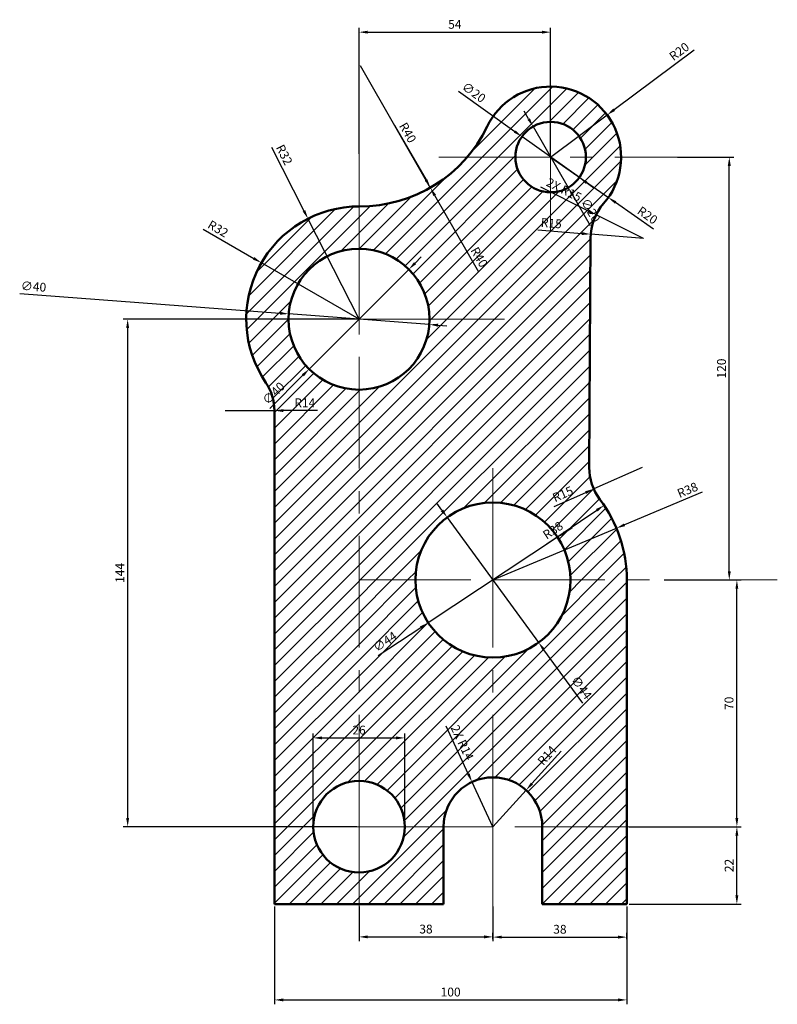
# Model space of a CAD drawing. Units: millimetres. Extents: x 2125 to 2340, y 1172 to 1452.
import ezdxf

# ---------------------------------------------------------------- set-up
doc = ezdxf.new("R2010")
doc.units = ezdxf.units.MM
doc.linetypes.add('CENTER', pattern=[50.8, 31.75, -6.35, 6.35, -6.35])
for name, color, linetype, lineweight in [('M-CNTR', 4, 'CENTER', 18), ('M-DIMS', 2, 'Continuous', 25), ('M-HATC', 8, 'Continuous', 18), ('M-OUTL', 7, 'Continuous', 50)]:
    doc.layers.add(name, color=color, linetype=linetype, lineweight=lineweight)
doc.styles.get("Standard").update_dxf_attribs({"font": 'arial.ttf'})
doc.dimstyles.new('ISO-25', dxfattribs={"dimtxt": 2.5, "dimasz": 2.5, "dimexe": 1.25, "dimexo": 0.625, "dimtad": 1, "dimdec": 0, "dimtxsty": 'Standard', "dimcen": 2.5, "dimadec": 0, "dimazin": 0, "dimtfac": 1, "dimtdec": 0, "dimtmove": 0, "dimatfit": 3, "dimfxl": 1, "dimarcsym": 0})

# ---------------------------------------------------------------- blocks, each defined once
blk = doc.blocks.new('*D1')
at = {"layer": 'Defpoints', "color": 0, "transparency": 16777216}
for p in [(2311.5, 1412.62), (2326.85, 1412.62), (2311.5, 1292.62)]:
    blk.add_point(p, dxfattribs=at)
at = {"layer": 'M-DIMS', "color": 0, "lineweight": -2, "transparency": 16777216}
for p, q in [((2312.12, 1412.62), (2328.1, 1412.62)), ((2326.85, 1295.12), (2326.85, 1410.12)), ((2312.12, 1292.62), (2328.1, 1292.62))]:
    blk.add_line(p, q, dxfattribs=at)
at = {"layer": 'M-DIMS', "color": 0, "transparency": 16777216}
for points in [[(2326.43, 1410.12), (2327.27, 1410.12), (2326.85, 1412.62)], [(2326.43, 1295.12), (2327.27, 1295.12), (2326.85, 1292.62)]]:
    blk.add_solid(points, dxfattribs=at)
at = {"layer": 'M-DIMS', "color": 0, "transparency": 16777216, "insert": (2324.95, 1352.62), "char_height": 2.5, "attachment_point": 5, "rotation": 90}
blk.add_mtext('120', dxfattribs=at)
blk = doc.blocks.new('*D2')
at = {"layer": 'Defpoints', "color": 0, "transparency": 16777216}
for p in [(2276.15, 1448.06), (2221.77, 1412.88), (2276.15, 1412.62)]:
    blk.add_point(p, dxfattribs=at)
at = {"layer": 'M-DIMS', "color": 0, "lineweight": -2, "transparency": 16777216}
for p, q in [((2221.77, 1413.51), (2221.77, 1449.31)), ((2224.27, 1448.06), (2273.65, 1448.06)), ((2276.15, 1413.24), (2276.15, 1449.31))]:
    blk.add_line(p, q, dxfattribs=at)
at = {"layer": 'M-DIMS', "color": 0, "transparency": 16777216}
for points in [[(2224.27, 1448.48), (2224.27, 1447.65), (2221.77, 1448.06)], [(2273.65, 1448.48), (2273.65, 1447.65), (2276.15, 1448.06)]]:
    blk.add_solid(points, dxfattribs=at)
at = {"layer": 'M-DIMS', "color": 0, "transparency": 16777216, "insert": (2248.96, 1449.96), "char_height": 2.5, "attachment_point": 5}
blk.add_mtext('54', dxfattribs=at)
blk = doc.blocks.new('*D3')
at = {"layer": 'Defpoints', "color": 0, "transparency": 16777216}
for p in [(2307.75, 1292.62), (2329, 1292.62), (2307.75, 1222.62)]:
    blk.add_point(p, dxfattribs=at)
at = {"layer": 'M-DIMS', "color": 0, "lineweight": -2, "transparency": 16777216}
for p, q in [((2308.38, 1292.62), (2330.25, 1292.62)), ((2329, 1225.12), (2329, 1290.12)), ((2308.38, 1222.62), (2330.25, 1222.62))]:
    blk.add_line(p, q, dxfattribs=at)
at = {"layer": 'M-DIMS', "color": 0, "transparency": 16777216}
for points in [[(2328.58, 1290.12), (2329.41, 1290.12), (2329, 1292.62)], [(2328.58, 1225.12), (2329.41, 1225.12), (2329, 1222.62)]]:
    blk.add_solid(points, dxfattribs=at)
at = {"layer": 'M-DIMS', "color": 0, "transparency": 16777216, "insert": (2327.09, 1257.62), "char_height": 2.5, "attachment_point": 5, "rotation": 90}
blk.add_mtext('70', dxfattribs=at)
blk = doc.blocks.new('*D4')
at = {"layer": 'Defpoints', "color": 0, "transparency": 16777216}
for p in [(2297.77, 1222.62), (2329, 1222.62), (2297.77, 1200.62)]:
    blk.add_point(p, dxfattribs=at)
at = {"layer": 'M-DIMS', "color": 0, "lineweight": -2, "transparency": 16777216}
for p, q in [((2298.39, 1222.62), (2330.25, 1222.62)), ((2329, 1203.12), (2329, 1220.12)), ((2298.39, 1200.62), (2330.25, 1200.62))]:
    blk.add_line(p, q, dxfattribs=at)
at = {"layer": 'M-DIMS', "color": 0, "transparency": 16777216}
for points in [[(2328.58, 1220.12), (2329.41, 1220.12), (2329, 1222.62)], [(2328.58, 1203.12), (2329.41, 1203.12), (2329, 1200.62)]]:
    blk.add_solid(points, dxfattribs=at)
at = {"layer": 'M-DIMS', "color": 0, "transparency": 16777216, "insert": (2327.12, 1211.62), "char_height": 2.5, "attachment_point": 5, "rotation": 90}
blk.add_mtext('22', dxfattribs=at)
blk = doc.blocks.new('*D5')
at = {"layer": 'Defpoints', "color": 0, "transparency": 16777216}
for p in [(2221.77, 1366.62), (2156.11, 1222.62), (2221.77, 1222.62)]:
    blk.add_point(p, dxfattribs=at)
at = {"layer": 'M-DIMS', "color": 0, "lineweight": -2, "transparency": 16777216}
for p, q in [((2221.14, 1366.62), (2154.86, 1366.62)), ((2156.11, 1364.12), (2156.11, 1225.12)), ((2221.14, 1222.62), (2154.86, 1222.62))]:
    blk.add_line(p, q, dxfattribs=at)
at = {"layer": 'M-DIMS', "color": 0, "transparency": 16777216}
for points in [[(2155.69, 1364.12), (2156.53, 1364.12), (2156.11, 1366.62)], [(2155.69, 1225.12), (2156.53, 1225.12), (2156.11, 1222.62)]]:
    blk.add_solid(points, dxfattribs=at)
at = {"layer": 'M-DIMS', "color": 0, "transparency": 16777216, "insert": (2154.23, 1294.62), "char_height": 2.5, "attachment_point": 5, "rotation": 90}
blk.add_mtext('144', dxfattribs=at)
blk = doc.blocks.new('*D6')
at = {"layer": 'Defpoints', "color": 0, "transparency": 16777216}
for p in [(2234.77, 1247.81), (2208.77, 1222.62), (2234.77, 1222.62)]:
    blk.add_point(p, dxfattribs=at)
at = {"layer": 'M-DIMS', "color": 0, "lineweight": -2, "transparency": 16777216}
for p, q in [((2208.77, 1223.24), (2208.77, 1249.06)), ((2234.77, 1223.24), (2234.77, 1249.06)), ((2211.27, 1247.81), (2232.27, 1247.81))]:
    blk.add_line(p, q, dxfattribs=at)
at = {"layer": 'M-DIMS', "color": 0, "transparency": 16777216}
for points in [[(2211.27, 1248.23), (2211.27, 1247.4), (2208.77, 1247.81)], [(2232.27, 1248.23), (2232.27, 1247.4), (2234.77, 1247.81)]]:
    blk.add_solid(points, dxfattribs=at)
at = {"layer": 'M-DIMS', "color": 0, "transparency": 16777216, "insert": (2221.77, 1249.71), "char_height": 2.5, "attachment_point": 5}
blk.add_mtext('26', dxfattribs=at)
blk = doc.blocks.new('*D7')
at = {"layer": 'Defpoints', "color": 0, "transparency": 16777216}
for p in [(2292.19, 1424.57), (2276.15, 1412.62)]:
    blk.add_point(p, dxfattribs=at)
at = {"layer": 'M-DIMS', "color": 0, "lineweight": -2, "transparency": 16777216}
for p, q in [((2316.85, 1442.95), (2294.19, 1426.06)), ((2276.15, 1412.62), (2292.19, 1424.57))]:
    blk.add_line(p, q, dxfattribs=at)
at = {"layer": 'M-DIMS', "color": 0, "transparency": 16777216}
blk.add_solid([(2293.94, 1426.4), (2294.44, 1425.73), (2292.19, 1424.57)], dxfattribs=at)
at = {"layer": 'M-DIMS', "color": 0, "transparency": 16777216, "insert": (2312.82, 1442.32), "char_height": 2.5, "attachment_point": 5, "rotation": 36.702}
blk.add_mtext('R20', dxfattribs=at)
blk = doc.blocks.new('*D8')
at = {"layer": 'Defpoints', "color": 0, "transparency": 16777216}
for p in [(2222.08, 1438.62), (2242.03, 1403.95)]:
    blk.add_point(p, dxfattribs=at)
at = {"layer": 'M-DIMS', "color": 0, "lineweight": -2, "transparency": 16777216}
blk.add_line((2231.88, 1421.58), (2240.79, 1406.12), dxfattribs=at)
at = {"layer": 'M-DIMS', "color": 0, "transparency": 16777216}
blk.add_solid([(2241.15, 1406.32), (2240.43, 1405.91), (2242.03, 1403.95)], dxfattribs=at)
at = {"layer": 'M-DIMS', "color": 0, "transparency": 16777216, "insert": (2235.33, 1419.4), "char_height": 2.5, "attachment_point": 5, "rotation": 299.9242}
blk.add_mtext('R40', dxfattribs=at)
blk = doc.blocks.new('*D9')
at = {"layer": 'Defpoints', "color": 0, "transparency": 16777216}
for p in [(2287.51, 1390.73), (2302.46, 1389.53)]:
    blk.add_point(p, dxfattribs=at)
at = {"layer": 'M-DIMS', "color": 0, "lineweight": -2, "transparency": 16777216}
for p, q in [((2272.54, 1391.93), (2285.02, 1390.93)), ((2302.46, 1389.53), (2287.51, 1390.73))]:
    blk.add_line(p, q, dxfattribs=at)
at = {"layer": 'M-DIMS', "color": 0, "transparency": 16777216}
blk.add_solid([(2285.05, 1391.34), (2284.98, 1390.51), (2287.51, 1390.73)], dxfattribs=at)
at = {"layer": 'M-DIMS', "color": 0, "transparency": 16777216, "insert": (2276.31, 1393.53), "char_height": 2.5, "attachment_point": 5, "rotation": 355.4193}
blk.add_mtext('R15', dxfattribs=at)
blk = doc.blocks.new('*D10')
at = {"layer": 'Defpoints', "color": 0, "transparency": 16777216}
for p in [(2302.1, 1324.5), (2288.38, 1318.44)]:
    blk.add_point(p, dxfattribs=at)
at = {"layer": 'M-DIMS', "color": 0, "lineweight": -2, "transparency": 16777216}
for p, q in [((2302.1, 1324.5), (2288.38, 1318.44)), ((2277.18, 1313.5), (2286.1, 1317.43))]:
    blk.add_line(p, q, dxfattribs=at)
at = {"layer": 'M-DIMS', "color": 0, "transparency": 16777216}
blk.add_solid([(2285.93, 1317.81), (2286.26, 1317.05), (2288.38, 1318.44)], dxfattribs=at)
at = {"layer": 'M-DIMS', "color": 0, "transparency": 16777216, "insert": (2279.73, 1316.7), "char_height": 2.5, "attachment_point": 5, "rotation": 23.827}
blk.add_mtext('R15', dxfattribs=at)
blk = doc.blocks.new('*D11')
at = {"layer": 'Defpoints', "color": 0, "transparency": 16777216}
for p in [(2291.32, 1313.8), (2259.77, 1292.62)]:
    blk.add_point(p, dxfattribs=at)
at = {"layer": 'M-DIMS', "color": 0, "lineweight": -2, "transparency": 16777216}
blk.add_line((2275.03, 1302.86), (2289.24, 1312.4), dxfattribs=at)
at = {"layer": 'M-DIMS', "color": 0, "transparency": 16777216}
blk.add_solid([(2289.01, 1312.75), (2289.48, 1312.06), (2291.32, 1313.8)], dxfattribs=at)
at = {"layer": 'M-DIMS', "color": 0, "transparency": 16777216, "insert": (2276.97, 1306.46), "char_height": 2.5, "attachment_point": 5, "rotation": 33.8706}
blk.add_mtext('R38', dxfattribs=at)
blk = doc.blocks.new('*D12')
at = {"layer": 'Defpoints', "color": 0, "transparency": 16777216}
for p in [(2194.06, 1382.62), (2221.77, 1366.62)]:
    blk.add_point(p, dxfattribs=at)
at = {"layer": 'M-DIMS', "color": 0, "lineweight": -2, "transparency": 16777216}
for p, q in [((2177.53, 1392.16), (2191.89, 1383.87)), ((2221.77, 1366.62), (2194.06, 1382.62))]:
    blk.add_line(p, q, dxfattribs=at)
at = {"layer": 'M-DIMS', "color": 0, "transparency": 16777216}
blk.add_solid([(2192.1, 1384.23), (2191.68, 1383.51), (2194.06, 1382.62)], dxfattribs=at)
at = {"layer": 'M-DIMS', "color": 0, "transparency": 16777216, "insert": (2181.6, 1392), "char_height": 2.5, "attachment_point": 5, "rotation": 330}
blk.add_mtext('R32', dxfattribs=at)
blk = doc.blocks.new('*D13')
at = {"layer": 'Defpoints', "color": 0, "transparency": 16777216}
for p in [(2183.77, 1340.69), (2197.77, 1340.69)]:
    blk.add_point(p, dxfattribs=at)
at = {"layer": 'M-DIMS', "color": 0, "lineweight": -2, "transparency": 16777216}
for p, q in [((2183.77, 1340.69), (2197.77, 1340.69)), ((2209.98, 1340.69), (2200.27, 1340.69))]:
    blk.add_line(p, q, dxfattribs=at)
at = {"layer": 'M-DIMS', "color": 0, "transparency": 16777216}
blk.add_solid([(2200.27, 1341.11), (2200.27, 1340.28), (2197.77, 1340.69)], dxfattribs=at)
at = {"layer": 'M-DIMS', "color": 0, "transparency": 16777216, "insert": (2206.38, 1342.57), "char_height": 2.5, "attachment_point": 5}
blk.add_mtext('R14', dxfattribs=at)
blk = doc.blocks.new('*D14')
at = {"layer": 'Defpoints', "color": 0, "transparency": 16777216}
for p in [(2269.17, 1232.99), (2259.77, 1222.62)]:
    blk.add_point(p, dxfattribs=at)
at = {"layer": 'M-DIMS', "color": 0, "lineweight": -2, "transparency": 16777216}
for p, q in [((2279.17, 1244.04), (2270.85, 1234.85)), ((2259.77, 1222.62), (2269.17, 1232.99))]:
    blk.add_line(p, q, dxfattribs=at)
at = {"layer": 'M-DIMS', "color": 0, "transparency": 16777216}
blk.add_solid([(2270.54, 1235.13), (2271.15, 1234.57), (2269.17, 1232.99)], dxfattribs=at)
at = {"layer": 'M-DIMS', "color": 0, "transparency": 16777216, "insert": (2275.36, 1242.63), "char_height": 2.5, "attachment_point": 5, "rotation": 47.8267}
blk.add_mtext('R14', dxfattribs=at)
blk = doc.blocks.new('*D15')
at = {"layer": 'Defpoints', "color": 0, "transparency": 16777216}
for p in [(2221.77, 1200.62), (2259.77, 1200.62), (2259.77, 1191.35)]:
    blk.add_point(p, dxfattribs=at)
at = {"layer": 'M-DIMS', "color": 0, "lineweight": -2, "transparency": 16777216}
for p, q in [((2221.77, 1199.99), (2221.77, 1190.1)), ((2259.77, 1199.99), (2259.77, 1190.1)), ((2224.27, 1191.35), (2257.27, 1191.35))]:
    blk.add_line(p, q, dxfattribs=at)
at = {"layer": 'M-DIMS', "color": 0, "transparency": 16777216}
for points in [[(2224.27, 1191.77), (2224.27, 1190.93), (2221.77, 1191.35)], [(2257.27, 1191.77), (2257.27, 1190.93), (2259.77, 1191.35)]]:
    blk.add_solid(points, dxfattribs=at)
at = {"layer": 'M-DIMS', "color": 0, "transparency": 16777216, "insert": (2240.77, 1193.25), "char_height": 2.5, "attachment_point": 5}
blk.add_mtext('38', dxfattribs=at)
blk = doc.blocks.new('*D16')
at = {"layer": 'Defpoints', "color": 0, "transparency": 16777216}
for p in [(2297.77, 1191.29), (2259.77, 1190.1), (2297.77, 1190.1)]:
    blk.add_point(p, dxfattribs=at)
at = {"layer": 'M-DIMS', "color": 0, "lineweight": -2, "transparency": 16777216}
for p, q in [((2259.77, 1190.73), (2259.77, 1192.54)), ((2262.27, 1191.29), (2295.27, 1191.29)), ((2297.77, 1190.73), (2297.77, 1192.54))]:
    blk.add_line(p, q, dxfattribs=at)
at = {"layer": 'M-DIMS', "color": 0, "transparency": 16777216}
for points in [[(2262.27, 1191.71), (2262.27, 1190.87), (2259.77, 1191.29)], [(2295.27, 1191.71), (2295.27, 1190.87), (2297.77, 1191.29)]]:
    blk.add_solid(points, dxfattribs=at)
at = {"layer": 'M-DIMS', "color": 0, "transparency": 16777216, "insert": (2278.77, 1193.19), "char_height": 2.5, "attachment_point": 5}
blk.add_mtext('38', dxfattribs=at)
blk = doc.blocks.new('*D17')
at = {"layer": 'Defpoints', "color": 0, "transparency": 16777216}
for p in [(2201.82, 1368.12), (2241.71, 1365.11)]:
    blk.add_point(p, dxfattribs=at)
at = {"layer": 'M-DIMS', "color": 0, "lineweight": -2, "transparency": 16777216}
for p, q in [((2125.47, 1373.88), (2199.33, 1368.31)), ((2241.71, 1365.11), (2201.82, 1368.12)), ((2244.2, 1364.92), (2246.7, 1364.74))]:
    blk.add_line(p, q, dxfattribs=at)
at = {"layer": 'M-DIMS', "color": 0, "transparency": 16777216}
for points in [[(2199.36, 1368.73), (2199.3, 1367.89), (2201.82, 1368.12)], [(2244.24, 1365.34), (2244.17, 1364.51), (2241.71, 1365.11)]]:
    blk.add_solid(points, dxfattribs=at)
at = {"layer": 'M-DIMS', "color": 0, "transparency": 16777216, "insert": (2129.38, 1375.57), "char_height": 2.5, "attachment_point": 5, "rotation": 355.6851}
blk.add_mtext('∅40', dxfattribs=at)
blk = doc.blocks.new('*D18')
at = {"layer": 'Defpoints', "color": 0, "transparency": 16777216}
for p in [(2246.78, 1310.38), (2272.75, 1274.86)]:
    blk.add_point(p, dxfattribs=at)
at = {"layer": 'M-DIMS', "color": 0, "lineweight": -2, "transparency": 16777216}
for p, q in [((2245.31, 1312.39), (2243.83, 1314.41)), ((2246.78, 1310.38), (2272.75, 1274.86)), ((2285.31, 1257.69), (2274.23, 1272.84))]:
    blk.add_line(p, q, dxfattribs=at)
at = {"layer": 'M-DIMS', "color": 0, "transparency": 16777216}
for points in [[(2245.64, 1312.64), (2244.97, 1312.15), (2246.78, 1310.38)], [(2274.56, 1273.09), (2273.89, 1272.59), (2272.75, 1274.86)]]:
    blk.add_solid(points, dxfattribs=at)
at = {"layer": 'M-DIMS', "color": 0, "transparency": 16777216, "insert": (2284.67, 1261.89), "char_height": 2.5, "attachment_point": 5, "rotation": 306.1722}
blk.add_mtext('∅44', dxfattribs=at)
blk = doc.blocks.new('*D19')
at = {"layer": 'Defpoints', "color": 0, "transparency": 16777216}
for p in [(2197.77, 1200.62), (2297.77, 1200.62), (2297.77, 1173.47)]:
    blk.add_point(p, dxfattribs=at)
at = {"layer": 'M-DIMS', "color": 0, "lineweight": -2, "transparency": 16777216}
for p, q in [((2197.77, 1199.99), (2197.77, 1172.22)), ((2297.77, 1199.99), (2297.77, 1172.22)), ((2200.27, 1173.47), (2295.27, 1173.47))]:
    blk.add_line(p, q, dxfattribs=at)
at = {"layer": 'M-DIMS', "color": 0, "transparency": 16777216}
for points in [[(2200.27, 1173.89), (2200.27, 1173.06), (2197.77, 1173.47)], [(2295.27, 1173.89), (2295.27, 1173.06), (2297.77, 1173.47)]]:
    blk.add_solid(points, dxfattribs=at)
at = {"layer": 'M-DIMS', "color": 0, "transparency": 16777216, "insert": (2247.77, 1175.38), "char_height": 2.5, "attachment_point": 5}
blk.add_mtext('100', dxfattribs=at)
blk = doc.blocks.new('*D20')
at = {"layer": 'Defpoints', "color": 0, "transparency": 16777216}
for p in [(2268.01, 1418.42), (2284.3, 1406.81)]:
    blk.add_point(p, dxfattribs=at)
at = {"layer": 'M-DIMS', "color": 0, "lineweight": -2, "transparency": 16777216}
for p, q in [((2249.96, 1431.3), (2265.98, 1419.87)), ((2284.3, 1406.81), (2268.01, 1418.42)), ((2286.33, 1405.36), (2288.37, 1403.91))]:
    blk.add_line(p, q, dxfattribs=at)
at = {"layer": 'M-DIMS', "color": 0, "transparency": 16777216}
for points in [[(2266.22, 1420.21), (2265.73, 1419.53), (2268.01, 1418.42)], [(2286.57, 1405.7), (2286.09, 1405.02), (2284.3, 1406.81)]]:
    blk.add_solid(points, dxfattribs=at)
at = {"layer": 'M-DIMS', "color": 0, "transparency": 16777216, "insert": (2254.17, 1430.71), "char_height": 2.5, "attachment_point": 5, "rotation": 324.511}
blk.add_mtext('∅20', dxfattribs=at)
blk = doc.blocks.new('*D21')
at = {"layer": 'Defpoints', "color": 0, "transparency": 16777216}
for p in [(2294.81, 1307.31), (2259.77, 1292.62)]:
    blk.add_point(p, dxfattribs=at)
at = {"layer": 'M-DIMS', "color": 0, "lineweight": -2, "transparency": 16777216}
for p, q in [((2319.18, 1317.52), (2297.12, 1308.27)), ((2259.77, 1292.62), (2294.81, 1307.31))]:
    blk.add_line(p, q, dxfattribs=at)
at = {"layer": 'M-DIMS', "color": 0, "transparency": 16777216}
blk.add_solid([(2296.96, 1308.66), (2297.28, 1307.89), (2294.81, 1307.31)], dxfattribs=at)
at = {"layer": 'M-DIMS', "color": 0, "transparency": 16777216, "insert": (2315.11, 1317.87), "char_height": 2.5, "attachment_point": 5, "rotation": 22.7399}
blk.add_mtext('R38', dxfattribs=at)
blk = doc.blocks.new('*D22')
at = {"layer": 'Defpoints', "color": 0, "transparency": 16777216}
for p in [(2207.28, 1395.15), (2221.77, 1366.62)]:
    blk.add_point(p, dxfattribs=at)
at = {"layer": 'M-DIMS', "color": 0, "lineweight": -2, "transparency": 16777216}
for p, q in [((2196.95, 1415.47), (2206.14, 1397.38)), ((2221.77, 1366.62), (2207.28, 1395.15))]:
    blk.add_line(p, q, dxfattribs=at)
at = {"layer": 'M-DIMS', "color": 0, "transparency": 16777216}
blk.add_solid([(2206.52, 1397.57), (2205.77, 1397.19), (2207.28, 1395.15)], dxfattribs=at)
at = {"layer": 'M-DIMS', "color": 0, "transparency": 16777216, "insert": (2200.28, 1413.13), "char_height": 2.5, "attachment_point": 5, "rotation": 296.929}
blk.add_mtext('R32', dxfattribs=at)
blk = doc.blocks.new('*D23')
at = {"layer": 'Defpoints', "color": 0, "transparency": 16777216}
for p in [(2278.13, 1304.74), (2241.41, 1280.5)]:
    blk.add_point(p, dxfattribs=at)
at = {"layer": 'M-DIMS', "color": 0, "lineweight": -2, "transparency": 16777216}
for p, q in [((2280.21, 1306.12), (2282.3, 1307.49)), ((2278.13, 1304.74), (2241.41, 1280.5)), ((2227.25, 1271.15), (2239.32, 1279.12))]:
    blk.add_line(p, q, dxfattribs=at)
at = {"layer": 'M-DIMS', "color": 0, "transparency": 16777216}
for points in [[(2279.98, 1306.46), (2280.44, 1305.77), (2278.13, 1304.74)], [(2239.09, 1279.47), (2239.55, 1278.77), (2241.41, 1280.5)]]:
    blk.add_solid(points, dxfattribs=at)
at = {"layer": 'M-DIMS', "color": 0, "transparency": 16777216, "insert": (2229.31, 1274.87), "char_height": 2.5, "attachment_point": 5, "rotation": 33.4335}
blk.add_mtext('∅44', dxfattribs=at)
blk = doc.blocks.new('*D24')
at = {"layer": 'Defpoints', "color": 0, "transparency": 16777216}
for p in [(2235.91, 1380.76), (2207.63, 1352.48)]:
    blk.add_point(p, dxfattribs=at)
at = {"layer": 'M-DIMS', "color": 0, "lineweight": -2, "transparency": 16777216}
for p, q in [((2237.68, 1382.53), (2239.45, 1384.29)), ((2235.91, 1380.76), (2207.63, 1352.48)), ((2196.47, 1341.32), (2205.86, 1350.71))]:
    blk.add_line(p, q, dxfattribs=at)
at = {"layer": 'M-DIMS', "color": 0, "transparency": 16777216}
for points in [[(2237.38, 1382.82), (2237.97, 1382.23), (2235.91, 1380.76)], [(2205.56, 1351), (2206.15, 1350.41), (2207.63, 1352.48)]]:
    blk.add_solid(points, dxfattribs=at)
at = {"layer": 'M-DIMS', "color": 0, "transparency": 16777216, "insert": (2197.75, 1345.38), "char_height": 2.5, "attachment_point": 5, "rotation": 44.998}
blk.add_mtext('∅40', dxfattribs=at)
blk = doc.blocks.new('*D25')
at = {"layer": 'Defpoints', "color": 0, "transparency": 16777216}
for p in [(2276.15, 1412.62), (2292.54, 1401.15)]:
    blk.add_point(p, dxfattribs=at)
at = {"layer": 'M-DIMS', "color": 0, "lineweight": -2, "transparency": 16777216}
for p, q in [((2276.15, 1412.62), (2292.54, 1401.15)), ((2305.33, 1392.2), (2294.59, 1399.72))]:
    blk.add_line(p, q, dxfattribs=at)
at = {"layer": 'M-DIMS', "color": 0, "transparency": 16777216}
blk.add_solid([(2294.83, 1400.06), (2294.35, 1399.38), (2292.54, 1401.15)], dxfattribs=at)
at = {"layer": 'M-DIMS', "color": 0, "transparency": 16777216, "insert": (2303.46, 1395.83), "char_height": 2.5, "attachment_point": 5, "rotation": 325.0144}
blk.add_mtext('R20', dxfattribs=at)
blk = doc.blocks.new('*D26')
at = {"layer": 'Defpoints', "color": 0, "transparency": 16777216}
for p in [(2289.06, 1396.27), (2302.46, 1389.53)]:
    blk.add_point(p, dxfattribs=at)
at = {"layer": 'M-DIMS', "color": 0, "lineweight": -2, "transparency": 16777216}
for p, q in [((2273.29, 1404.2), (2286.83, 1397.39)), ((2302.46, 1389.53), (2289.06, 1396.27))]:
    blk.add_line(p, q, dxfattribs=at)
at = {"layer": 'M-DIMS', "color": 0, "transparency": 16777216}
blk.add_solid([(2287.01, 1397.77), (2286.64, 1397.02), (2289.06, 1396.27)], dxfattribs=at)
at = {"layer": 'M-DIMS', "color": 0, "transparency": 16777216, "insert": (2279.79, 1403.06), "char_height": 2.5, "attachment_point": 5, "rotation": 333.2984}
blk.add_mtext('2X R15', dxfattribs=at)
blk = doc.blocks.new('*D27')
at = {"layer": 'Defpoints', "color": 0, "transparency": 16777216}
for p in [(2253.85, 1235.3), (2259.77, 1222.62)]:
    blk.add_point(p, dxfattribs=at)
at = {"layer": 'M-DIMS', "color": 0, "lineweight": -2, "transparency": 16777216}
for p, q in [((2246.4, 1251.28), (2252.79, 1237.57)), ((2259.77, 1222.62), (2253.85, 1235.3))]:
    blk.add_line(p, q, dxfattribs=at)
at = {"layer": 'M-DIMS', "color": 0, "transparency": 16777216}
blk.add_solid([(2253.17, 1237.75), (2252.42, 1237.39), (2253.85, 1235.3)], dxfattribs=at)
at = {"layer": 'M-DIMS', "color": 0, "transparency": 16777216, "insert": (2250.77, 1246.35), "char_height": 2.5, "attachment_point": 5, "rotation": 295.007}
blk.add_mtext('2X R14', dxfattribs=at)
blk = doc.blocks.new('*D28')
at = {"layer": 'Defpoints', "color": 0, "transparency": 16777216}
for p in [(2271.16, 1421.28), (2281.15, 1403.96)]:
    blk.add_point(p, dxfattribs=at)
at = {"layer": 'M-DIMS', "color": 0, "lineweight": -2, "transparency": 16777216}
for p, q in [((2269.91, 1423.44), (2268.66, 1425.61)), ((2271.16, 1421.28), (2281.15, 1403.96)), ((2287.42, 1393.09), (2282.4, 1401.79))]:
    blk.add_line(p, q, dxfattribs=at)
at = {"layer": 'M-DIMS', "color": 0, "transparency": 16777216}
for points in [[(2270.27, 1423.65), (2269.55, 1423.24), (2271.16, 1421.28)], [(2282.76, 1402), (2282.04, 1401.58), (2281.15, 1403.96)]]:
    blk.add_solid(points, dxfattribs=at)
at = {"layer": 'M-DIMS', "color": 0, "transparency": 16777216, "insert": (2287.24, 1397.34), "char_height": 2.5, "attachment_point": 5, "rotation": 299.9873}
blk.add_mtext('∅20', dxfattribs=at)
blk = doc.blocks.new('*D29')
at = {"layer": 'Defpoints', "color": 0, "transparency": 16777216}
for p in [(2222.08, 1438.62), (2242, 1403.93)]:
    blk.add_point(p, dxfattribs=at)
at = {"layer": 'M-DIMS', "color": 0, "lineweight": -2, "transparency": 16777216}
for p, q in [((2222.08, 1438.62), (2242, 1403.93)), ((2255.75, 1379.99), (2243.24, 1401.76))]:
    blk.add_line(p, q, dxfattribs=at)
at = {"layer": 'M-DIMS', "color": 0, "transparency": 16777216}
blk.add_solid([(2243.6, 1401.97), (2242.88, 1401.55), (2242, 1403.93)], dxfattribs=at)
at = {"layer": 'M-DIMS', "color": 0, "transparency": 16777216, "insert": (2255.6, 1384.06), "char_height": 2.5, "attachment_point": 5, "rotation": 299.8652}
blk.add_mtext('R40', dxfattribs=at)

msp = doc.modelspace()

# ---------------------------------------------------------------- hatches: boundary and pattern name
at = {"layer": 'M-HATC'}
h = msp.add_hatch(dxfattribs=at)
h.set_pattern_fill('ANSI31', color=256)
h.paths.add_polyline_path([(2287.46, 1389.61, -0.180646), (2291.19, 1399.42, 0.182056), (2296.15, 1412.62), (2286.15, 1412.62, -1), (2266.15, 1412.62), (2252.48, 1412.62, -0.221265), (2221.77, 1398.62), (2221.77, 1386.62, -0.414214), (2241.77, 1366.62, -0.414214), (2221.77, 1346.62), (2221.77, 1292.62), (2237.77, 1292.62, -1), (2281.77, 1292.62), (2297.77, 1292.62, 0.16279), (2290.12, 1315.48, -0.164192), (2287.1, 1324.58)])
h.paths.add_polyline_path([(2276.15, 1432.62), (2276.15, 1422.62, -0.414214), (2286.15, 1412.62), (2296.15, 1412.62, 0.414214)])
h.paths.add_polyline_path([(2276.15, 1432.62, 0.288264), (2258.13, 1421.28, -0.064938), (2252.48, 1412.62), (2266.15, 1412.62, -0.414214), (2276.15, 1422.62)])
h.paths.add_polyline_path([(2201.77, 1366.62), (2189.77, 1366.62, 0.150795), (2195.33, 1348.58, -0.150795), (2197.77, 1340.69), (2197.77, 1222.62), (2208.77, 1222.62, -0.414214), (2221.77, 1235.62), (2221.77, 1346.62, -0.414214)])
h.paths.add_polyline_path([(2221.77, 1386.62), (2221.77, 1398.62, 0.414214), (2189.77, 1366.62), (2201.77, 1366.62, -0.414214)])
h = msp.add_hatch(dxfattribs=at)
h.set_pattern_fill('ANSI31', color=256)
h.paths.add_polyline_path([(2297.77, 1292.62), (2281.77, 1292.62, -0.414214), (2259.77, 1270.62), (2259.77, 1236.62, -0.414214), (2273.77, 1222.62), (2297.77, 1222.62)])
h.paths.add_polyline_path([(2259.77, 1270.62, -0.414214), (2237.77, 1292.62), (2221.77, 1292.62), (2221.77, 1235.62, -0.414214), (2234.77, 1222.62), (2245.77, 1222.62, -0.414214), (2259.77, 1236.62)])
h.paths.add_polyline_path([(2208.77, 1222.62), (2197.77, 1222.62), (2197.77, 1200.62), (2201.77, 1200.62), (2221.77, 1200.62), (2221.77, 1209.62, -0.414214)])
h.paths.add_polyline_path([(2245.77, 1222.62), (2234.77, 1222.62, -0.414214), (2221.77, 1209.62), (2221.77, 1200.62), (2245.77, 1200.62)])
h.paths.add_polyline_path([(2297.77, 1222.62), (2273.77, 1222.62), (2273.77, 1200.62), (2297.77, 1200.62)])

# ---------------------------------------------------------------- linework, layer by layer
at = {"layer": 'M-CNTR'}
for p, q in [((2276.15, 1412.62), (2276.15, 1448.1)), ((2221.77, 1386.61), (2221.77, 1439.16)), ((2276.15, 1412.62), (2241.11, 1412.62)), ((2326.15, 1412.62), (2276.15, 1412.62)), ((2276.15, 1412.62), (2276.15, 1391.73)), ((2221.77, 1366.62), (2221.77, 1386.61)), ((2202.75, 1366.62), (2171.57, 1366.62)), ((2246.31, 1366.62), (2202.75, 1366.62)), ((2221.77, 1222.62), (2221.77, 1366.62)), ((2221.77, 1366.62), (2246.31, 1366.62)), ((2246.31, 1366.62), (2263.09, 1366.62)), ((2259.77, 1292.62), (2259.77, 1326.89)), ((2221.77, 1292.62), (2259.77, 1292.62)), ((2259.77, 1222.62), (2259.77, 1292.62)), ((2259.77, 1292.62), (2297.25, 1292.62)), ((2259.77, 1292.62), (2340.48, 1292.62)), ((2221.77, 1222.62), (2189.81, 1222.62)), ((2208.77, 1222.62), (2197.77, 1222.62)), ((2208.77, 1222.62), (2197.77, 1222.62)), ((2221.77, 1222.62), (2210.77, 1222.62)), ((2221.77, 1222.62), (2210.77, 1222.62)), ((2297.77, 1222.62), (2221.77, 1222.62)), ((2259.77, 1222.62), (2221.77, 1222.62)), ((2221.77, 1222.62), (2221.77, 1190.05)), ((2259.77, 1222.62), (2259.77, 1200.62)), ((2297.77, 1222.62), (2317.74, 1222.62)), ((2259.77, 1200.62), (2259.77, 1198.08))]:
    msp.add_line(p, q, dxfattribs=at)
at = {"layer": 'M-OUTL'}
for p, q in [((2287.46, 1389.61), (2287.1, 1324.58)), ((2197.77, 1222.62), (2197.77, 1340.69)), ((2297.77, 1222.62), (2297.77, 1292.62)), ((2197.77, 1222.62), (2197.77, 1200.62)), ((2245.77, 1222.62), (2245.77, 1200.62)), ((2273.77, 1222.62), (2273.77, 1200.62)), ((2297.77, 1200.62), (2297.77, 1222.62)), ((2201.77, 1200.62), (2197.77, 1200.62)), ((2201.77, 1200.62), (2245.77, 1200.62)), ((2273.77, 1200.62), (2297.77, 1200.62))]:
    msp.add_line(p, q, dxfattribs=at)
for centre, radius in [((2276.15, 1412.62), 10), ((2221.77, 1366.62), 20), ((2259.77, 1292.62), 22), ((2221.77, 1222.62), 13)]:
    msp.add_circle(centre, radius, dxfattribs=at)
for centre, radius, start, end in [((2276.15, 1412.62), 20, 318.7278, 154.3214), ((2222.08, 1438.62), 40, 269.752, 334.3214), ((2221.77, 1366.62), 32, 89.752, 214.3012), ((2302.46, 1389.53), 15, 138.7278, 179.6871), ((2183.77, 1340.69), 14, 0, 34.3012), ((2302.1, 1324.5), 15, 179.6871, 216.9843), ((2259.77, 1292.62), 38, 0, 36.9843), ((2259.77, 1222.62), 14, 0, 180)]:
    msp.add_arc(centre, radius, start, end, dxfattribs=at)

# ---------------------------------------------------------------- dimensions: what is measured, and where the dimension line sits
at = {"layer": 'M-DIMS'}
dim = msp.add_linear_dim(base=(2276.15, 1448.06), p1=(2221.77, 1412.88), p2=(2276.15, 1412.62), dimstyle='ISO-25', override={"dimclrd": 0, "dimclre": 0, "dimclrt": 0}, dxfattribs=at)
dim.commit()
dim.dimension.update_dxf_attribs({"geometry": '*D2', "text_midpoint": (2248.96, 1449.96)})
for center, mpoint, override, picture, middle in [((2276.15, 1412.62), (2292.19, 1424.57), {"dimclrd": 0, "dimclre": 0, "dimclrt": 0}, '*D7', (2313.95, 1440.79)), ((2222.08, 1438.62), (2242.03, 1403.95), {"dimclrd": 0, "dimclre": 0, "dimclrt": 0}, '*D8', (2233.68, 1418.46)), ((2222.08, 1438.62), (2242, 1403.93), {"dimdec": 0, "dimlfac": 1, "dimrnd": 0, "dimzin": 0, "dimdsep": 46, "dimlunit": 2}, '*D29', (2253.95, 1383.12)), ((2221.77, 1366.62), (2207.28, 1395.15), {"dimdec": 0, "dimlfac": 1, "dimrnd": 0, "dimzin": 0, "dimdsep": 46, "dimlunit": 2}, '*D22', (2198.58, 1412.27)), ((2276.15, 1412.62), (2292.54, 1401.15), {"dimdec": 0, "dimlfac": 1, "dimrnd": 0, "dimzin": 0, "dimdsep": 46, "dimlunit": 2}, '*D25', (2302.37, 1394.27)), ((2221.77, 1366.62), (2194.06, 1382.62), {"dimclrd": 0, "dimclre": 0, "dimclrt": 0}, '*D12', (2180.65, 1390.36)), ((2302.46, 1389.53), (2287.51, 1390.73), {"dimclrd": 0, "dimclre": 0, "dimclrt": 0}, '*D9', (2276.15, 1391.64)), ((2259.77, 1292.62), (2294.81, 1307.31), {"dimdec": 0, "dimlfac": 1, "dimrnd": 0, "dimzin": 0, "dimdsep": 46, "dimlunit": 2}, '*D21', (2315.84, 1316.12)), ((2259.77, 1292.62), (2291.32, 1313.8), {"dimclrd": 0, "dimclre": 0, "dimclrt": 0}, '*D11', (2278.03, 1304.88)), ((2259.77, 1222.62), (2269.17, 1232.99), {"dimclrd": 0, "dimclre": 0, "dimclrt": 0}, '*D14', (2276.75, 1241.36))]:
    dim = msp.add_radius_dim(center=center, mpoint=mpoint, dimstyle='ISO-25', override=override, dxfattribs=at)
    dim.commit()
    dim.dimension.update_dxf_attribs({"geometry": picture, "text_midpoint": middle, "dimtype": 164})
for p1, p2, override, picture, middle in [((2284.3, 1406.81), (2268.01, 1418.42), {"dimclrd": 0, "dimclre": 0, "dimclrt": 0}, '*D20', (2253.03, 1429.11)), ((2271.16, 1421.28), (2281.15, 1403.96), {"dimdec": 0, "dimlfac": 1, "dimrnd": 0, "dimzin": 0, "dimdsep": 46, "dimlunit": 2}, '*D28', (2285.54, 1396.36)), ((2235.91, 1380.76), (2207.63, 1352.48), {"dimdec": 0, "dimlfac": 1, "dimrnd": 0, "dimzin": 0, "dimdsep": 46, "dimlunit": 2}, '*D24', (2199.14, 1343.99)), ((2241.71, 1365.11), (2201.82, 1368.12), {"dimclrd": 0, "dimclre": 0, "dimclrt": 0}, '*D17', (2129.23, 1373.6)), ((2246.78, 1310.38), (2272.75, 1274.86), {"dimclrd": 0, "dimclre": 0, "dimclrt": 0}, '*D18', (2283.08, 1260.73)), ((2278.13, 1304.74), (2241.41, 1280.5), {"dimdec": 0, "dimlfac": 1, "dimrnd": 0, "dimzin": 0, "dimdsep": 46, "dimlunit": 2}, '*D23', (2230.39, 1273.22))]:
    dim = msp.add_diameter_dim_2p(p1=p1, p2=p2, dimstyle='ISO-25', override=override, dxfattribs=at)
    dim.commit()
    dim.dimension.update_dxf_attribs({"geometry": picture, "text_midpoint": middle, "dimtype": 163})
dim = msp.add_linear_dim(base=(2326.85, 1412.62), p1=(2311.5, 1292.62), p2=(2311.5, 1412.62), angle=90, dimstyle='ISO-25', override={"dimclrd": 0, "dimclre": 0, "dimclrt": 0}, dxfattribs=at)
dim.commit()
dim.dimension.update_dxf_attribs({"geometry": '*D1', "text_midpoint": (2326.85, 1352.62), "dimtype": 160})
for center, mpoint, picture, middle in [((2302.46, 1389.53), (2289.06, 1396.27), '*D26', (2279.79, 1403.06)), ((2259.77, 1222.62), (2253.85, 1235.3), '*D27', (2250.77, 1246.35))]:
    dim = msp.add_radius_dim(center=center, mpoint=mpoint, text='2X <>', dimstyle='ISO-25', override={"dimdec": 0, "dimlfac": 1, "dimrnd": 0, "dimzin": 0, "dimdsep": 46, "dimlunit": 2}, dxfattribs=at)
    dim.commit()
    dim.dimension.update_dxf_attribs({"geometry": picture, "text_midpoint": middle})
for p1, p2, distance, picture, middle in [((2221.77, 1366.62), (2221.77, 1222.62), -65.66, '*D5', (2154.23, 1294.62)), ((2307.75, 1222.62), (2307.75, 1292.62), -21.24, '*D3', (2327.09, 1257.62)), ((2208.77, 1222.62), (2234.77, 1222.62), 25.19, '*D6', (2221.77, 1249.71)), ((2297.77, 1200.62), (2297.77, 1222.62), -31.23, '*D4', (2327.12, 1211.62)), ((2197.77, 1200.62), (2297.77, 1200.62), -27.14, '*D19', (2247.77, 1175.38)), ((2221.77, 1200.62), (2259.77, 1200.62), -9.27, '*D15', (2240.77, 1193.25)), ((2259.77, 1190.1), (2297.77, 1190.1), 1.19, '*D16', (2278.77, 1193.19))]:
    dim = msp.add_aligned_dim(p1=p1, p2=p2, distance=distance, dimstyle='ISO-25', override={"dimclrd": 0, "dimclre": 0, "dimclrt": 0}, dxfattribs=at)
    dim.commit()
    dim.dimension.update_dxf_attribs({"geometry": picture, "text_midpoint": middle})
for center, mpoint, picture, middle in [((2183.77, 1340.69), (2197.77, 1340.69), '*D13', (2206.38, 1342.57)), ((2302.1, 1324.5), (2288.38, 1318.44), '*D10', (2279.73, 1316.7))]:
    dim = msp.add_radius_dim(center=center, mpoint=mpoint, dimstyle='ISO-25', override={"dimclrd": 0, "dimclre": 0, "dimclrt": 0}, dxfattribs=at)
    dim.commit()
    dim.dimension.update_dxf_attribs({"geometry": picture, "text_midpoint": middle})

doc.saveas('drawing.dxf')
